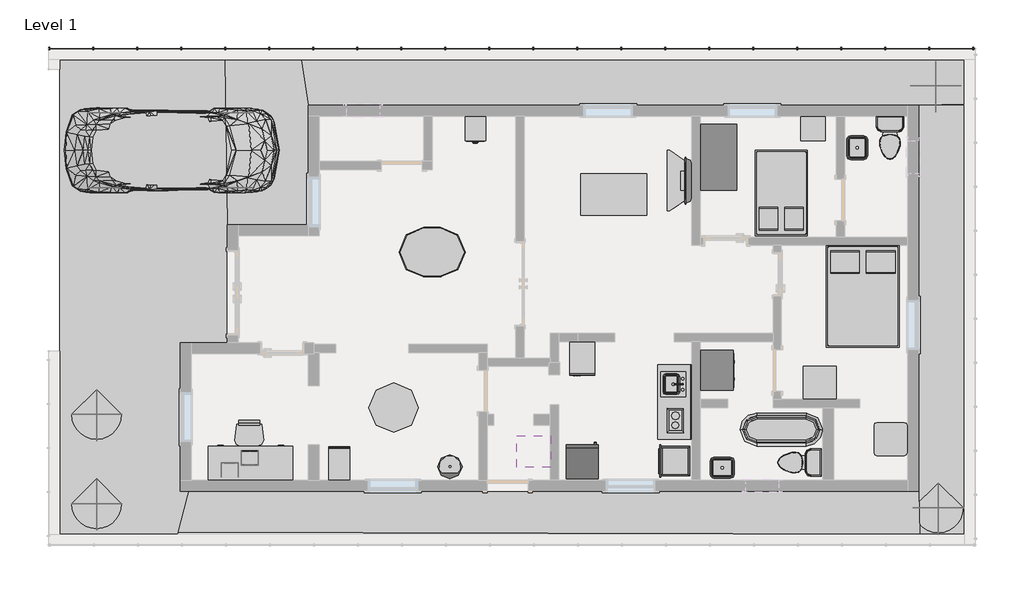
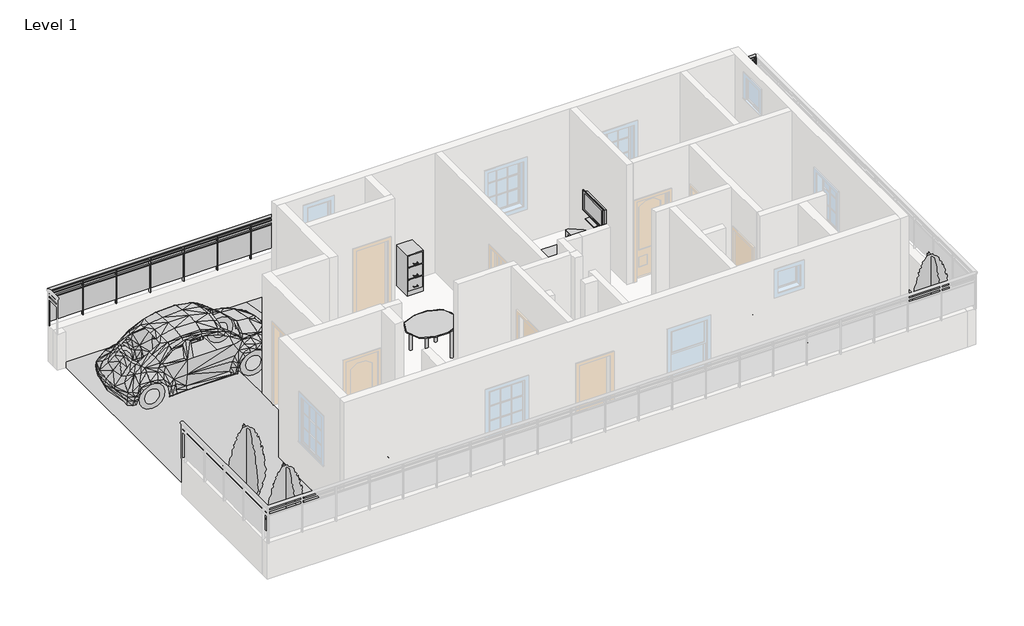
# One storey, part 3 of 3: 16 furniture elements, 15 proxies, 7 flow terminals, 4 geographic elements, 1 railing.
"""IFC4 building model written with IfcOpenShell, lengths in millimetres."""

from ifc_helpers import new_model, si_unit, point, frame, origin, place, context, project, spatial, polyline, ellipse_curve, trimmed, outline, extrude, triangles, transform, mapped, element, save
from ifc_brep_helpers import plane_surface, extruded_surface, advanced_brep
from components import entourage_4c8cfd20, proxy_db4bb64d, proxy_7e1014cc, proxy_fe84b772, proxy_a6faaae8, proxy_844211aa, proxy_8b8c2dc4, rpc_beetle_rpc_beetle_3ce7ba48, proxy_c523a7b7, flow_terminal_871c2e40, flow_terminal_d49f872f, flow_terminal_62a433f7, toilet_domestic_3d_toilet_domestic_3d_f7549cf7, toilet_domestic_3d_toilet_domestic_3d_183bbd19, flow_terminal_2ffd2f66, furniture_c8abb964, furniture_631c00ae, furniture_552c1472, chair_desk_chair_desk_ccc35c8f, furniture_b3f308bd, furniture_072f6425, furniture_08c10487, furniture_80f2079a, furniture_56245f3a, tv_stand_tv_stand_6ce107e5, furniture_e3bc833e, furniture_be1c6672, furniture_905aceb5, furniture_bcf351fa, furniture_097b63cf, furniture_5bc9ed15, rpc_tree_conifer_0001_chinese_juniper_7_1b9786cd

model = new_model("IFC4")

# Units and contexts
model_context = context("Model", 3, world=origin())
ifc_project = project(units=[si_unit("LENGTHUNIT", "METRE", prefix="MILLI")], contexts=[model_context])

# Site, building, storey
site = spatial("IfcSite", under=ifc_project)
building = spatial("IfcBuilding", under=site)
storey = spatial("IfcBuildingStorey", under=building, Name="Level 1", Elevation=0.0)

# Proxies
placement = place(None, origin())
element("IfcBuildingElementProxy", 1, Name="Building Element Proxy", at=placement, inside=storey, context=model_context, shape_type="Tessellation", body=[
    triangles([(-21898.1191772, 12173.6662354, 0.0), (-21898.1191772, 3410.6659447, 0.0), (-19722.5659241, 3410.6659447, 0.0), (-19666.685614, 6966.0811935, 0.0), (-19748.6015442, 10092.3002563, 0.0), (-18803.0848389, 6966.0811935, 0.0), (-18803.0848389, 9125.0813873, 0.0), (-18943.9727509, 10074.8350433, 0.0), (-18848.4588135, 12173.6662354, 0.0)], [[4, 1, 2], [1, 5, 9], [4, 5, 1], [2, 3, 4], [4, 6, 7], [6, 4, 3], [8, 7, 9], [8, 5, 7], [9, 5, 8], [5, 4, 7]], closed=False),
])
element("IfcBuildingElementProxy", 2, Name="Building Element Proxy", at=placement, inside=storey, context=model_context, shape_type="Tessellation", body=[
    triangles([(-18803.0848389, 9125.0813873, 0.0), (-17304.4844513, 9125.0813873, 0.0), (-17304.4844513, 11334.8813873, 0.0), (-17434.4451233, 12173.6662354, 0.0), (-18907.1703461, 12173.6662354, 0.0)], [[5, 1, 3], [5, 3, 4], [3, 1, 2]], closed=False),
])
element("IfcBuildingElementProxy", 3, Name="Building Element Proxy", at=placement, inside=storey, context=model_context, shape_type="Tessellation", body=[
    triangles([(-17304.4844513, 11334.8813873, 0.0), (-17438.9181061, 12173.6662354, 0.0), (-5184.9201462, 12173.6662354, 0.0), (-6026.8844513, 11334.8813873, 0.0), (-5184.9201462, 11344.9063568, 0.0)], [[2, 1, 4], [4, 5, 3], [4, 3, 2]], closed=False),
])
element("IfcBuildingElementProxy", 4, Name="Building Element Proxy", at=placement, inside=storey, context=model_context, shape_type="Tessellation", body=[
    triangles([(-5184.9201462, 11341.3716888, 0.0), (-6026.8844513, 11334.8813873, 0.0), (-6023.0718933, 3410.6659447, 0.0), (-5184.9201462, 3410.6659447, 0.0)], [[2, 3, 4], [4, 1, 2]], closed=False),
])
element("IfcBuildingElementProxy", 5, Name="Building Element Proxy", at=placement, inside=storey, context=model_context, shape_type="Tessellation", body=[
    triangles([(-19541.1653687, 4197.4812904, 0.0), (-19710.431781, 3439.8970093, 0.0), (-6026.8844513, 4197.4812904, 0.0), (-6033.6526428, 3410.6659447, 0.0), (-6026.8396866, 3410.6659447, 0.0), (-6011.1662247, 3410.6659447, 0.0), (-6028.8971191, 3410.6659447, 0.0)], [[2, 4, 1], [1, 4, 3], [5, 6, 3], [7, 3, 4], [3, 7, 5]], closed=False),
])
entourage_shape = entourage_4c8cfd20(model_context)
element("IfcBuildingElementProxy", 6, Name="Entourage", at=placement, inside=storey, context=model_context, shape_type="MappedRepresentation", body=[
    mapped(entourage_shape, transform((-18757.4020483, 4629.2812219, 0.0), x_axis=(1.0, 0.0, 0.0), y_axis=(0.0, 1.0, 0.0), z_axis=(0.0, 0.0, 1.0))),
])
element("IfcBuildingElementProxy", 7, Name="Entourage", at=placement, inside=storey, context=model_context, shape_type="MappedRepresentation", body=[
    mapped(entourage_shape, transform((-18387.2011117, 4781.6812219, 762.0), x_axis=(-1.0000000000000004, 0.0, 0.0), y_axis=(0.0, -1.0000000000000004, 0.0), z_axis=(0.0, 0.0, 1.0))),
])
proxy_shape = proxy_db4bb64d(model_context)
element("IfcBuildingElementProxy", 8, Name="15\" x 24\" x 34 1/2\"", ObjectType="15\" x 24\" x 34 1/2\"", at=placement, inside=storey, context=model_context, shape_type="MappedRepresentation", body=[
    mapped(proxy_shape, transform((-16464.9670881, 4969.5328437, 0.0), x_axis=(-1.0, 0.0, 0.0), y_axis=(0.0, -1.0, 0.0), z_axis=(0.0, 0.0, 1.0))),
])
proxy_2_shape = proxy_7e1014cc(model_context)
element("IfcBuildingElementProxy", 9, Name="18\" x 24\" x 34 1/2\"", ObjectType="18\" x 24\" x 34 1/2\"", at=placement, inside=storey, context=model_context, shape_type="MappedRepresentation", body=[
    mapped(proxy_2_shape, transform((-12549.6520251, 6394.8316571, 0.0), x_axis=(1.0, 0.0, 0.0), y_axis=(0.0, 1.0, 0.0), z_axis=(0.0, 0.0, 1.0))),
])
proxy_3_shape = proxy_fe84b772(model_context)
element("IfcBuildingElementProxy", 10, Name="Cook Top-2 Unit : 12\" x 18\"", ObjectType="Cook Top-2 Unit : 12\" x 18\"", at=placement, inside=storey, context=model_context, shape_type="MappedRepresentation", body=[
    mapped(proxy_3_shape, transform((-10598.8845566, 5475.3564263, 0.0), x_axis=(1.0, 0.0, 0.0), y_axis=(0.0, 1.0, 0.0), z_axis=(0.0, 0.0, 1.0))),
])
proxy_4_shape = proxy_a6faaae8(model_context)
element("IfcBuildingElementProxy", 11, Name="Cook Top-4 Unit2 : 22\" x 20\"", ObjectType="Cook Top-4 Unit2 : 22\" x 20\"", at=placement, inside=storey, context=model_context, shape_type="MappedRepresentation", body=[
    mapped(proxy_4_shape, transform((-13138.8845566, 4934.0812219, 914.4), x_axis=(1.0, 0.0, 0.0), y_axis=(0.0, 1.0, 0.0), z_axis=(0.0, 0.0, 1.0))),
])
proxy_5_shape = proxy_844211aa(model_context)
element("IfcBuildingElementProxy", 12, Name="Kitchenette - Small : 54\"", ObjectType="Kitchenette - Small : 54\"", at=placement, inside=storey, context=model_context, shape_type="MappedRepresentation", body=[
    mapped(proxy_5_shape, transform((-10217.8845566, 5867.2189268, 0.0), x_axis=(0.0, -1.0, 0.0), y_axis=(1.0, 0.0, 0.0), z_axis=(0.0, 0.0, 1.0))),
])
proxy_6_shape = proxy_8b8c2dc4(model_context)
element("IfcBuildingElementProxy", 13, Name="Oven Double-Built-in : 21 1/2\" x 39 1/4\" x 21\"", ObjectType="Oven Double-Built-in : 21 1/2\" x 39 1/4\" x 21\"", at=placement, inside=storey, context=model_context, shape_type="MappedRepresentation", body=[
    mapped(proxy_6_shape, transform((-10663.7504156, 4721.1062946, 0.0), x_axis=(0.0, -1.0000000000000004, 0.0), y_axis=(1.0000000000000004, 0.0, 0.0), z_axis=(0.0, 0.0, 1.0))),
])
rpc_beetle_rpc_beetle_shape = rpc_beetle_rpc_beetle_3ce7ba48(model_context)
element("IfcBuildingElementProxy", 14, Name="RPC Beetle : RPC Beetle", ObjectType="RPC Beetle : RPC Beetle", at=placement, inside=storey, context=model_context, shape_type="MappedRepresentation", body=[
    mapped(rpc_beetle_rpc_beetle_shape, transform((-21063.6845566, 10496.6812219, 0.0), x_axis=(0.0, -1.0000000000000002, 0.0), y_axis=(1.0000000000000002, 0.0, 0.0), z_axis=(0.0, 0.0, 1.0))),
])
proxy_7_shape = proxy_c523a7b7(model_context)
element("IfcBuildingElementProxy", 15, Name="Refrigerator : 24\" x 25\" LH", ObjectType="Refrigerator : 24\" x 25\" LH", at=placement, inside=storey, context=model_context, shape_type="MappedRepresentation", body=[
    mapped(proxy_7_shape, transform((-12243.5345566, 4729.6822504, 0.0), x_axis=(-1.0000000000000004, 0.0, 0.0), y_axis=(0.0, -1.0000000000000004, 0.0), z_axis=(0.0, 0.0, 1.0))),
])

# Flow terminals
flow_terminal_shape = flow_terminal_871c2e40(model_context)
element("IfcFlowTerminal", 16, ObjectType="Sink Kitchen-Island : 18\" x 18\"", at=placement, inside=storey, context=model_context, shape_type="MappedRepresentation", body=[
    mapped(flow_terminal_shape, transform((-10563.1299577, 6194.3704625, 0.0), x_axis=(0.0, -1.0, 0.0), y_axis=(1.0, 0.0, 0.0), z_axis=(0.0, 0.0, 1.0))),
])
flow_terminal_2_shape = flow_terminal_d49f872f(model_context)
element("IfcFlowTerminal", 17, ObjectType="Sink Vanity-Round : 19\" x 19\"", at=placement, inside=storey, context=model_context, shape_type="MappedRepresentation", body=[
    mapped(flow_terminal_2_shape, transform((-14591.632816, 4740.1488915, 482.6), x_axis=(-1.0000000000000004, 0.0, 0.0), y_axis=(0.0, -1.0000000000000004, 0.0), z_axis=(0.0, 0.0, 1.0))),
])
flow_terminal_3_shape = flow_terminal_62a433f7(model_context)
element("IfcFlowTerminal", 18, ObjectType="Sink Vanity-Square : 20\" x 18\"", at=placement, inside=storey, context=model_context, shape_type="MappedRepresentation", body=[
    mapped(flow_terminal_3_shape, transform((-9643.395316, 4580.826623, 609.6), x_axis=(-1.0000000000000002, 0.0, 0.0), y_axis=(0.0, -1.0000000000000002, 0.0), z_axis=(0.0, 0.0, 1.0))),
])
element("IfcFlowTerminal", 19, ObjectType="Sink Vanity-Square : 20\" x 18\"", at=placement, inside=storey, context=model_context, shape_type="MappedRepresentation", body=[
    mapped(flow_terminal_3_shape, transform((-7218.3391555, 10531.7919813, 609.6), x_axis=(0.0, 1.0000000000000004, 0.0), y_axis=(-1.0000000000000004, 0.0, 0.0), z_axis=(0.0, 0.0, 1.0))),
])
toilet_domestic_3d_toilet_domestic_3d_shape = toilet_domestic_3d_toilet_domestic_3d_f7549cf7(model_context)
toilet_domestic_3d_toilet_domestic_3d_2_shape = toilet_domestic_3d_toilet_domestic_3d_183bbd19(model_context)
element("IfcFlowTerminal", 20, ObjectType="Toilet-Domestic-3D : Toilet-Domestic-3D", at=placement, inside=storey, context=model_context, shape_type="MappedRepresentation", body=[
    mapped(toilet_domestic_3d_toilet_domestic_3d_shape, transform((-8324.980584, 4730.8812219, 0.0), x_axis=(0.0, -1.0000000000000004, 0.0), y_axis=(1.0000000000000004, 0.0, 0.0), z_axis=(0.0, 0.0, 1.0))),
    mapped(toilet_domestic_3d_toilet_domestic_3d_2_shape, transform((-8324.980584, 4730.8812219, 0.0), x_axis=(0.0, -1.0000000000000004, 0.0), y_axis=(1.0000000000000004, 0.0, 0.0), z_axis=(0.0, 0.0, 1.0))),
])
element("IfcFlowTerminal", 21, ObjectType="Toilet-Domestic-3D : Toilet-Domestic-3D", at=placement, inside=storey, context=model_context, shape_type="MappedRepresentation", body=[
    mapped(toilet_domestic_3d_toilet_domestic_3d_shape, transform((-6560.2845566, 10636.9851945, 0.0), x_axis=(1.0, 0.0, 0.0), y_axis=(0.0, 1.0, 0.0), z_axis=(0.0, 0.0, 1.0))),
    mapped(toilet_domestic_3d_toilet_domestic_3d_2_shape, transform((-6560.2845566, 10636.9851945, 0.0), x_axis=(1.0, 0.0, 0.0), y_axis=(0.0, 1.0, 0.0), z_axis=(0.0, 0.0, 1.0))),
])
flow_terminal_4_shape = flow_terminal_2ffd2f66(model_context)
element("IfcFlowTerminal", 22, ObjectType="Tub-Free Standing-3D : 30\" x 60\"", at=placement, inside=storey, context=model_context, shape_type="MappedRepresentation", body=[
    mapped(flow_terminal_4_shape, transform((-8566.8845566, 5340.4812219, 0.0), x_axis=(0.0, -0.9999999999999998, 0.0), y_axis=(0.9999999999999998, 0.0, 0.0), z_axis=(0.0, 0.0, 1.0))),
])

# Furniture
furniture_shape = furniture_c8abb964(model_context)
element("IfcFurniture", 23, ObjectType="Bed-Box : Double 53\" x 74\"", at=placement, inside=storey, context=model_context, shape_type="MappedRepresentation", body=[
    mapped(furniture_shape, transform((-7398.4845566, 8038.7107301, 0.0), x_axis=(1.0, 0.0, 0.0), y_axis=(0.0, 1.0, 0.0), z_axis=(0.0, 0.0, 1.0))),
])
furniture_2_shape = furniture_631c00ae(model_context)
element("IfcFurniture", 24, ObjectType="Bed-Box : Twin 38\" x 74\"", at=placement, inside=storey, context=model_context, shape_type="MappedRepresentation", body=[
    mapped(furniture_2_shape, transform((-8227.7320976, 9474.8517137, 0.0), x_axis=(-1.0, 0.0, 0.0), y_axis=(0.0, -1.0, 0.0), z_axis=(0.0, 0.0, 1.0))),
])
furniture_3_shape = furniture_552c1472(model_context)
element("IfcFurniture", 25, ObjectType="Cabinet-File 3 Drawer : 15\" x 18\"", at=placement, inside=storey, context=model_context, shape_type="MappedRepresentation", body=[
    mapped(furniture_3_shape, transform((-14090.4881096, 11045.215522, 0.0), x_axis=(1.0, 0.0, 0.0), y_axis=(0.0, 1.0, 0.0), z_axis=(0.0, 0.0, 1.0))),
])
chair_desk_chair_desk_shape = chair_desk_chair_desk_ccc35c8f(model_context)
element("IfcFurniture", 26, ObjectType="Chair-Desk : Chair-Desk", at=placement, inside=storey, context=model_context, shape_type="MappedRepresentation", body=[
    mapped(chair_desk_chair_desk_shape, transform((-18396.6845566, 5442.0812219, 0.0), x_axis=(-1.0, 0.0, 0.0), y_axis=(0.0, -1.0, 0.0), z_axis=(0.0, 0.0, 1.0))),
])
furniture_4_shape = furniture_b3f308bd(model_context)
element("IfcFurniture", 27, ObjectType="Counter Top w Sink Hole : 24\" Depth", at=placement, inside=storey, context=model_context, shape_type="MappedRepresentation", body=[
    mapped(furniture_4_shape, transform((-10217.8845566, 5333.8189268, 0.0), x_axis=(0.0, -1.0, 0.0), y_axis=(1.0, 0.0, 0.0), z_axis=(0.0, 0.0, 1.0))),
])
furniture_5_shape = furniture_072f6425(model_context)
element("IfcFurniture", 28, ObjectType="Desk : 60\" x 30\"", at=placement, inside=storey, context=model_context, shape_type="MappedRepresentation", body=[
    mapped(furniture_5_shape, transform((-19133.2845566, 4248.2812219, 0.0), x_axis=(1.0000000000000007, 0.0, 0.0), y_axis=(0.0, 1.0000000000000007, 0.0), z_axis=(0.0, 0.0, 1.0))),
])
furniture_6_shape = furniture_08c10487(model_context)
element("IfcFurniture", 29, ObjectType="Dresser.0001 : 48\" x 60\" x 24\"", at=placement, inside=storey, context=model_context, shape_type="MappedRepresentation", body=[
    mapped(furniture_6_shape, transform((-10123.8475107, 6701.8744817, 0.0), x_axis=(0.0, 1.0000000000000002, 0.0), y_axis=(-1.0000000000000002, 0.0, 0.0), z_axis=(0.0, 0.0, 1.0))),
])
furniture_7_shape = furniture_80f2079a(model_context)
element("IfcFurniture", 30, ObjectType="Entertainment Center : 72\" x 72\" x 24\"", at=placement, inside=storey, context=model_context, shape_type="MappedRepresentation", body=[
    mapped(furniture_7_shape, transform((-10167.0845566, 10369.6812219, 0.0), x_axis=(0.0, 1.0000000000000002, 0.0), y_axis=(-1.0000000000000002, 0.0, 0.0), z_axis=(0.0, 0.0, 1.0))),
])
furniture_8_shape = furniture_56245f3a(model_context)
element("IfcFurniture", 31, ObjectType="TV - Flat Screen : 32\"", at=placement, inside=storey, context=model_context, shape_type="MappedRepresentation", body=[
    mapped(furniture_8_shape, transform((-10276.4231803, 9933.9367078, 914.4), x_axis=(0.0, -1.0000000000000002, 0.0), y_axis=(1.0000000000000002, 0.0, 0.0), z_axis=(0.0, 0.0, 1.0))),
])
tv_stand_tv_stand_shape = tv_stand_tv_stand_6ce107e5(model_context)
element("IfcFurniture", 32, ObjectType="TV Stand : TV Stand", at=placement, inside=storey, context=model_context, shape_type="MappedRepresentation", body=[
    mapped(tv_stand_tv_stand_shape, transform((-10217.8845566, 10063.069224, 0.0), x_axis=(0.0, -1.0000000000000004, 0.0), y_axis=(1.0000000000000004, 0.0, 0.0), z_axis=(0.0, 0.0, 1.0))),
])
furniture_9_shape = furniture_e3bc833e(model_context)
element("IfcFurniture", 33, ObjectType="Table-Dining : 30\" x 84\" x 22\"", at=placement, inside=storey, context=model_context, shape_type="MappedRepresentation", body=[
    mapped(furniture_9_shape, transform((-11683.9503233, 9588.6701441, 0.0), x_axis=(1.0, 0.0, 0.0), y_axis=(0.0, 1.0, 0.0), z_axis=(0.0, 0.0, 1.0))),
])
furniture_10_shape = furniture_be1c6672(model_context)
element("IfcFurniture", 34, ObjectType="Table-Dining Oval : 36\" x 48\"", at=placement, inside=storey, context=model_context, shape_type="MappedRepresentation", body=[
    mapped(furniture_10_shape, transform((-14616.6648845, 8975.1795826, 0.0), x_axis=(1.0, 0.0, 0.0), y_axis=(0.0, 1.0, 0.0), z_axis=(0.0, 0.0, 1.0))),
])
furniture_11_shape = furniture_905aceb5(model_context)
element("IfcFurniture", 35, ObjectType="Table-Dining Round w Chairs : 36\" Diameter", at=placement, inside=storey, context=model_context, shape_type="MappedRepresentation", body=[
    mapped(furniture_11_shape, transform((-15833.3665238, 5931.7599104, 0.0), x_axis=(1.0, 0.0, 0.0), y_axis=(0.0, 1.0, 0.0), z_axis=(0.0, 0.0, 1.0))),
])
furniture_12_shape = furniture_bcf351fa(model_context)
element("IfcFurniture", 36, ObjectType="Table-End : 24\" x 24\"", at=placement, inside=storey, context=model_context, shape_type="MappedRepresentation", body=[
    mapped(furniture_12_shape, transform((-6856.1181869, 5010.2812219, 0.0), x_axis=(1.0, 0.0, 0.0), y_axis=(0.0, 1.0, 0.0), z_axis=(0.0, 0.0, 1.0))),
])
furniture_13_shape = furniture_097b63cf(model_context)
element("IfcFurniture", 37, ObjectType="Table-Night Stand : 18\" x 18\" x 24\"", at=placement, inside=storey, context=model_context, shape_type="MappedRepresentation", body=[
    mapped(furniture_13_shape, transform((-8215.0181869, 10674.4812219, 0.0), x_axis=(1.0, 0.0, 0.0), y_axis=(0.0, 1.0, 0.0), z_axis=(0.0, 0.0, 1.0))),
])
furniture_14_shape = furniture_5bc9ed15(model_context)
element("IfcFurniture", 38, ObjectType="Table-Night Stand : 24\" x 24\" x 30\"", at=placement, inside=storey, context=model_context, shape_type="MappedRepresentation", body=[
    mapped(furniture_14_shape, transform((-8164.2181869, 5899.2812219, 0.0), x_axis=(1.0, 0.0, 0.0), y_axis=(0.0, 1.0, 0.0), z_axis=(0.0, 0.0, 1.0))),
])

# Geographic elements
rpc_tree_conifer_0001_chinese_juniper_7_shape = rpc_tree_conifer_0001_chinese_juniper_7_1b9786cd(model_context)
element("IfcGeographicElement", 39, ObjectType="RPC Tree - Conifer.0001 : Chinese Juniper - 7'", at=placement, inside=storey, context=model_context, shape_type="MappedRepresentation", body=[
    mapped(rpc_tree_conifer_0001_chinese_juniper_7_shape, transform((-21216.2812277, 3968.8812219, 0.0), x_axis=(1.0, 0.0, 0.0), y_axis=(0.0, 1.0, 0.0), z_axis=(0.0, 0.0, 1.0))),
])
element("IfcGeographicElement", 40, ObjectType="RPC Tree - Conifer.0001 : Chinese Juniper - 7'", at=placement, inside=storey, context=model_context, shape_type="MappedRepresentation", body=[
    mapped(rpc_tree_conifer_0001_chinese_juniper_7_shape, transform((-21216.2812277, 5619.8812219, 0.0), x_axis=(1.0, 0.0, 0.0), y_axis=(0.0, 1.0, 0.0), z_axis=(0.0, 0.0, 1.0))),
])
element("IfcGeographicElement", 41, ObjectType="RPC Tree - Conifer.0001 : Chinese Juniper - 7'", at=placement, inside=storey, context=model_context, shape_type="MappedRepresentation", body=[
    mapped(rpc_tree_conifer_0001_chinese_juniper_7_shape, transform((-5667.7169317, 3892.6812219, 0.0), x_axis=(1.0, 0.0, 0.0), y_axis=(0.0, 1.0, 0.0), z_axis=(0.0, 0.0, 1.0))),
])
element("IfcGeographicElement", 42, ObjectType="RPC Tree - Conifer.0001 : Chinese Juniper - 7'", at=placement, inside=storey, context=model_context, shape_type="MappedRepresentation", body=[
    mapped(rpc_tree_conifer_0001_chinese_juniper_7_shape, transform((-5718.5169317, 11691.0658827, 0.0), x_axis=(1.0, 0.0, 0.0), y_axis=(0.0, 1.0, 0.0), z_axis=(0.0, 0.0, 1.0))),
])

# Railing
element("IfcRailing", 43, ObjectType="Glass Panel - Bottom Fill", at=placement, inside=storey, context=model_context, shape_type="SolidModel", body=[
    advanced_brep(
    [(-5007.1202606, 12338.7658827, 1828.8), (-5007.1202606, 12414.9658827, 1828.8), (-22101.3202606, 12338.7658827, 1828.8), (-22101.3202606, 12414.9658827, 1828.8)],
    [
        (0, 1, ellipse_curve(frame((-5007.1202606, 12376.8658827, 1828.8), z_axis=(1.0, 0.0, 0.0), x_axis=(0.0, 1.0, 0.0)), 38.1, 28.575)),
        (1, 0, ellipse_curve(frame((-5007.1202606, 12376.8658827, 1828.8), z_axis=(1.0, 0.0, 0.0), x_axis=(0.0, 1.0, 0.0)), 38.1, 28.575)),
        (2, 3, ellipse_curve(frame((-22101.3202606, 12376.8658827, 1828.8), z_axis=(-1.0, 0.0, 0.0), x_axis=(0.0, 1.0, 0.0)), 38.1, 28.575)),
        (3, 2, ellipse_curve(frame((-22101.3202606, 12376.8658827, 1828.8), z_axis=(-1.0, 0.0, 0.0), x_axis=(0.0, 1.0, 0.0)), 38.1, 28.575)),
        (0, 2),
        (3, 1),
    ],
    [
        plane_surface(frame((-5007.1202606, 12376.8658827, 1828.8), z_axis=(1.0, 0.0, 0.0), x_axis=(0.0, -1.0, 0.0))),
        plane_surface(frame((-22101.3202606, 12376.8658827, 1828.8), z_axis=(-1.0, 0.0, 0.0), x_axis=(0.0, -1.0, 0.0))),
        extruded_surface(trimmed(ellipse_curve(frame((-22101.3202606, 12376.8658827, 1828.8), z_axis=(1.0, 0.0, 0.0), x_axis=(0.0, 1.0, 0.0)), 38.1, 28.575), [point((-22101.3202606, 12338.7658827, 1828.8))], [point((-22101.3202606, 12414.9658827, 1828.8))], True, "CARTESIAN"), (17094.2, 0.0, 0.0), 17094.2),
        extruded_surface(trimmed(ellipse_curve(frame((-22101.3202606, 12376.8658827, 1828.8), z_axis=(1.0, 0.0, 0.0), x_axis=(0.0, 1.0, 0.0)), 38.1, 28.575), [point((-22101.3202606, 12414.9658827, 1828.8))], [point((-22101.3202606, 12338.7658827, 1828.8))], True, "CARTESIAN"), (17094.2, 0.0, 0.0), 17094.2),
    ],
    [
        (0, [[1, 2]]),
        (1, [[3, 4]]),
        (2, [[-1, 5, -4, 6]]),
        (3, [[-2, -6, -3, -5]]),
    ],
),
    extrude(outline(polyline([(-5007.1202606, 12389.5658827), (-5007.1202606, 12364.1658827), (-22101.3202606, 12364.1658827), (-22101.3202606, 12389.5658827), (-5007.1202606, 12389.5658827)])), frame((0.0, 0.0, 1714.5), z_axis=(0.0, 0.0, 1.0), x_axis=(1.0, 0.0, 0.0)), (0.0, 0.0, 1.0), 25.4),
    extrude(outline(polyline([(-5007.1202606, 12389.5658827), (-5007.1202606, 12364.1658827), (-22101.3202606, 12364.1658827), (-22101.3202606, 12389.5658827), (-5007.1202606, 12389.5658827)])), frame((0.0, 0.0, 1612.9), z_axis=(0.0, 0.0, 1.0), x_axis=(1.0, 0.0, 0.0)), (0.0, 0.0, 1.0), 25.4),
    extrude(outline(polyline([(-22082.2702606, 12402.2658827), (-22082.2702606, 12351.4658827), (-22094.9702606, 12351.4658827), (-22094.9702606, 12402.2658827), (-22082.2702606, 12402.2658827)])), frame((0.0, 0.0, 914.4), z_axis=(0.0, 0.0, 1.0), x_axis=(1.0, 0.0, 0.0)), (0.0, 0.0, 1.0), 885.6788223),
    extrude(outline(polyline([(-21275.8202606, 12370.3307257), (-22088.6202606, 12370.3307257), (-22088.6202606, 12376.6807257), (-21275.8202606, 12376.6807257), (-21275.8202606, 12370.3307257)])), frame((0.0, 0.0, 1016.0), z_axis=(0.0, 0.0, 1.0), x_axis=(1.0, 0.0, 0.0)), (0.0, 0.0, 1.0), 596.9),
    extrude(outline(polyline([(-21269.4702606, 12402.2658827), (-21269.4702606, 12351.4658827), (-21282.1702606, 12351.4658827), (-21282.1702606, 12402.2658827), (-21269.4702606, 12402.2658827)])), frame((0.0, 0.0, 914.4), z_axis=(0.0, 0.0, 1.0), x_axis=(1.0, 0.0, 0.0)), (0.0, 0.0, 1.0), 885.6788223),
    extrude(outline(polyline([(-20463.0202606, 12370.3307257), (-21275.8202606, 12370.3307257), (-21275.8202606, 12376.6807257), (-20463.0202606, 12376.6807257), (-20463.0202606, 12370.3307257)])), frame((0.0, 0.0, 1016.0), z_axis=(0.0, 0.0, 1.0), x_axis=(1.0, 0.0, 0.0)), (0.0, 0.0, 1.0), 596.9),
    extrude(outline(polyline([(-20456.6702606, 12402.2658827), (-20456.6702606, 12351.4658827), (-20469.3702606, 12351.4658827), (-20469.3702606, 12402.2658827), (-20456.6702606, 12402.2658827)])), frame((0.0, 0.0, 914.4), z_axis=(0.0, 0.0, 1.0), x_axis=(1.0, 0.0, 0.0)), (0.0, 0.0, 1.0), 885.6788223),
    extrude(outline(polyline([(-19650.2202606, 12370.3307257), (-20463.0202606, 12370.3307257), (-20463.0202606, 12376.6807257), (-19650.2202606, 12376.6807257), (-19650.2202606, 12370.3307257)])), frame((0.0, 0.0, 1016.0), z_axis=(0.0, 0.0, 1.0), x_axis=(1.0, 0.0, 0.0)), (0.0, 0.0, 1.0), 596.9),
    extrude(outline(polyline([(-19643.8702606, 12402.2658827), (-19643.8702606, 12351.4658827), (-19656.5702606, 12351.4658827), (-19656.5702606, 12402.2658827), (-19643.8702606, 12402.2658827)])), frame((0.0, 0.0, 914.4), z_axis=(0.0, 0.0, 1.0), x_axis=(1.0, 0.0, 0.0)), (0.0, 0.0, 1.0), 885.6788223),
    extrude(outline(polyline([(-18837.4202606, 12370.3307257), (-19650.2202606, 12370.3307257), (-19650.2202606, 12376.6807257), (-18837.4202606, 12376.6807257), (-18837.4202606, 12370.3307257)])), frame((0.0, 0.0, 1016.0), z_axis=(0.0, 0.0, 1.0), x_axis=(1.0, 0.0, 0.0)), (0.0, 0.0, 1.0), 596.9),
    extrude(outline(polyline([(-18831.0702606, 12402.2658827), (-18831.0702606, 12351.4658827), (-18843.7702606, 12351.4658827), (-18843.7702606, 12402.2658827), (-18831.0702606, 12402.2658827)])), frame((0.0, 0.0, 914.4), z_axis=(0.0, 0.0, 1.0), x_axis=(1.0, 0.0, 0.0)), (0.0, 0.0, 1.0), 885.6788223),
    extrude(outline(polyline([(-18024.6202606, 12370.3307257), (-18837.4202606, 12370.3307257), (-18837.4202606, 12376.6807257), (-18024.6202606, 12376.6807257), (-18024.6202606, 12370.3307257)])), frame((0.0, 0.0, 1016.0), z_axis=(0.0, 0.0, 1.0), x_axis=(1.0, 0.0, 0.0)), (0.0, 0.0, 1.0), 596.9),
    extrude(outline(polyline([(-18018.2702606, 12402.2658827), (-18018.2702606, 12351.4658827), (-18030.9702606, 12351.4658827), (-18030.9702606, 12402.2658827), (-18018.2702606, 12402.2658827)])), frame((0.0, 0.0, 914.4), z_axis=(0.0, 0.0, 1.0), x_axis=(1.0, 0.0, 0.0)), (0.0, 0.0, 1.0), 885.6788223),
    extrude(outline(polyline([(-17211.8202606, 12370.3307257), (-18024.6202606, 12370.3307257), (-18024.6202606, 12376.6807257), (-17211.8202606, 12376.6807257), (-17211.8202606, 12370.3307257)])), frame((0.0, 0.0, 1016.0), z_axis=(0.0, 0.0, 1.0), x_axis=(1.0, 0.0, 0.0)), (0.0, 0.0, 1.0), 596.9),
    extrude(outline(polyline([(-17205.4702606, 12402.2658827), (-17205.4702606, 12351.4658827), (-17218.1702606, 12351.4658827), (-17218.1702606, 12402.2658827), (-17205.4702606, 12402.2658827)])), frame((0.0, 0.0, 914.4), z_axis=(0.0, 0.0, 1.0), x_axis=(1.0, 0.0, 0.0)), (0.0, 0.0, 1.0), 885.6788223),
    extrude(outline(polyline([(-16399.0202606, 12370.3307257), (-17211.8202606, 12370.3307257), (-17211.8202606, 12376.6807257), (-16399.0202606, 12376.6807257), (-16399.0202606, 12370.3307257)])), frame((0.0, 0.0, 1016.0), z_axis=(0.0, 0.0, 1.0), x_axis=(1.0, 0.0, 0.0)), (0.0, 0.0, 1.0), 596.9),
    extrude(outline(polyline([(-16392.6702606, 12402.2658827), (-16392.6702606, 12351.4658827), (-16405.3702606, 12351.4658827), (-16405.3702606, 12402.2658827), (-16392.6702606, 12402.2658827)])), frame((0.0, 0.0, 914.4), z_axis=(0.0, 0.0, 1.0), x_axis=(1.0, 0.0, 0.0)), (0.0, 0.0, 1.0), 885.6788223),
    extrude(outline(polyline([(-15586.2202606, 12370.3307257), (-16399.0202606, 12370.3307257), (-16399.0202606, 12376.6807257), (-15586.2202606, 12376.6807257), (-15586.2202606, 12370.3307257)])), frame((0.0, 0.0, 1016.0), z_axis=(0.0, 0.0, 1.0), x_axis=(1.0, 0.0, 0.0)), (0.0, 0.0, 1.0), 596.9),
    extrude(outline(polyline([(-15579.8702606, 12402.2658827), (-15579.8702606, 12351.4658827), (-15592.5702606, 12351.4658827), (-15592.5702606, 12402.2658827), (-15579.8702606, 12402.2658827)])), frame((0.0, 0.0, 914.4), z_axis=(0.0, 0.0, 1.0), x_axis=(1.0, 0.0, 0.0)), (0.0, 0.0, 1.0), 885.6788223),
    extrude(outline(polyline([(-14773.4202606, 12370.3307257), (-15586.2202606, 12370.3307257), (-15586.2202606, 12376.6807257), (-14773.4202606, 12376.6807257), (-14773.4202606, 12370.3307257)])), frame((0.0, 0.0, 1016.0), z_axis=(0.0, 0.0, 1.0), x_axis=(1.0, 0.0, 0.0)), (0.0, 0.0, 1.0), 596.9),
    extrude(outline(polyline([(-14767.0702606, 12402.2658827), (-14767.0702606, 12351.4658827), (-14779.7702606, 12351.4658827), (-14779.7702606, 12402.2658827), (-14767.0702606, 12402.2658827)])), frame((0.0, 0.0, 914.4), z_axis=(0.0, 0.0, 1.0), x_axis=(1.0, 0.0, 0.0)), (0.0, 0.0, 1.0), 885.6788223),
    extrude(outline(polyline([(-13960.6202606, 12370.3307257), (-14773.4202606, 12370.3307257), (-14773.4202606, 12376.6807257), (-13960.6202606, 12376.6807257), (-13960.6202606, 12370.3307257)])), frame((0.0, 0.0, 1016.0), z_axis=(0.0, 0.0, 1.0), x_axis=(1.0, 0.0, 0.0)), (0.0, 0.0, 1.0), 596.9),
    extrude(outline(polyline([(-13954.2702606, 12402.2658827), (-13954.2702606, 12351.4658827), (-13966.9702606, 12351.4658827), (-13966.9702606, 12402.2658827), (-13954.2702606, 12402.2658827)])), frame((0.0, 0.0, 914.4), z_axis=(0.0, 0.0, 1.0), x_axis=(1.0, 0.0, 0.0)), (0.0, 0.0, 1.0), 885.6788223),
    extrude(outline(polyline([(-13147.8202606, 12370.3307257), (-13960.6202606, 12370.3307257), (-13960.6202606, 12376.6807257), (-13147.8202606, 12376.6807257), (-13147.8202606, 12370.3307257)])), frame((0.0, 0.0, 1016.0), z_axis=(0.0, 0.0, 1.0), x_axis=(1.0, 0.0, 0.0)), (0.0, 0.0, 1.0), 596.9),
    extrude(outline(polyline([(-13141.4702606, 12402.2658827), (-13141.4702606, 12351.4658827), (-13154.1702606, 12351.4658827), (-13154.1702606, 12402.2658827), (-13141.4702606, 12402.2658827)])), frame((0.0, 0.0, 914.4), z_axis=(0.0, 0.0, 1.0), x_axis=(1.0, 0.0, 0.0)), (0.0, 0.0, 1.0), 885.6788223),
    extrude(outline(polyline([(-12335.0202606, 12370.3307257), (-13147.8202606, 12370.3307257), (-13147.8202606, 12376.6807257), (-12335.0202606, 12376.6807257), (-12335.0202606, 12370.3307257)])), frame((0.0, 0.0, 1016.0), z_axis=(0.0, 0.0, 1.0), x_axis=(1.0, 0.0, 0.0)), (0.0, 0.0, 1.0), 596.9),
    extrude(outline(polyline([(-12328.6702606, 12402.2658827), (-12328.6702606, 12351.4658827), (-12341.3702606, 12351.4658827), (-12341.3702606, 12402.2658827), (-12328.6702606, 12402.2658827)])), frame((0.0, 0.0, 914.4), z_axis=(0.0, 0.0, 1.0), x_axis=(1.0, 0.0, 0.0)), (0.0, 0.0, 1.0), 885.6788223),
    extrude(outline(polyline([(-11522.2202606, 12370.3307257), (-12335.0202606, 12370.3307257), (-12335.0202606, 12376.6807257), (-11522.2202606, 12376.6807257), (-11522.2202606, 12370.3307257)])), frame((0.0, 0.0, 1016.0), z_axis=(0.0, 0.0, 1.0), x_axis=(1.0, 0.0, 0.0)), (0.0, 0.0, 1.0), 596.9),
    extrude(outline(polyline([(-11515.8702606, 12402.2658827), (-11515.8702606, 12351.4658827), (-11528.5702606, 12351.4658827), (-11528.5702606, 12402.2658827), (-11515.8702606, 12402.2658827)])), frame((0.0, 0.0, 914.4), z_axis=(0.0, 0.0, 1.0), x_axis=(1.0, 0.0, 0.0)), (0.0, 0.0, 1.0), 885.6788223),
    extrude(outline(polyline([(-10709.4202606, 12370.3307257), (-11522.2202606, 12370.3307257), (-11522.2202606, 12376.6807257), (-10709.4202606, 12376.6807257), (-10709.4202606, 12370.3307257)])), frame((0.0, 0.0, 1016.0), z_axis=(0.0, 0.0, 1.0), x_axis=(1.0, 0.0, 0.0)), (0.0, 0.0, 1.0), 596.9),
    extrude(outline(polyline([(-10703.0702606, 12402.2658827), (-10703.0702606, 12351.4658827), (-10715.7702606, 12351.4658827), (-10715.7702606, 12402.2658827), (-10703.0702606, 12402.2658827)])), frame((0.0, 0.0, 914.4), z_axis=(0.0, 0.0, 1.0), x_axis=(1.0, 0.0, 0.0)), (0.0, 0.0, 1.0), 885.6788223),
    extrude(outline(polyline([(-9896.6202606, 12370.3307257), (-10709.4202606, 12370.3307257), (-10709.4202606, 12376.6807257), (-9896.6202606, 12376.6807257), (-9896.6202606, 12370.3307257)])), frame((0.0, 0.0, 1016.0), z_axis=(0.0, 0.0, 1.0), x_axis=(1.0, 0.0, 0.0)), (0.0, 0.0, 1.0), 596.9),
    extrude(outline(polyline([(-9890.2702606, 12402.2658827), (-9890.2702606, 12351.4658827), (-9902.9702606, 12351.4658827), (-9902.9702606, 12402.2658827), (-9890.2702606, 12402.2658827)])), frame((0.0, 0.0, 914.4), z_axis=(0.0, 0.0, 1.0), x_axis=(1.0, 0.0, 0.0)), (0.0, 0.0, 1.0), 885.6788223),
    extrude(outline(polyline([(-9083.8202606, 12370.3307257), (-9896.6202606, 12370.3307257), (-9896.6202606, 12376.6807257), (-9083.8202606, 12376.6807257), (-9083.8202606, 12370.3307257)])), frame((0.0, 0.0, 1016.0), z_axis=(0.0, 0.0, 1.0), x_axis=(1.0, 0.0, 0.0)), (0.0, 0.0, 1.0), 596.9),
    extrude(outline(polyline([(-9077.4702606, 12402.2658827), (-9077.4702606, 12351.4658827), (-9090.1702606, 12351.4658827), (-9090.1702606, 12402.2658827), (-9077.4702606, 12402.2658827)])), frame((0.0, 0.0, 914.4), z_axis=(0.0, 0.0, 1.0), x_axis=(1.0, 0.0, 0.0)), (0.0, 0.0, 1.0), 885.6788223),
    extrude(outline(polyline([(-8271.0202606, 12370.3307257), (-9083.8202606, 12370.3307257), (-9083.8202606, 12376.6807257), (-8271.0202606, 12376.6807257), (-8271.0202606, 12370.3307257)])), frame((0.0, 0.0, 1016.0), z_axis=(0.0, 0.0, 1.0), x_axis=(1.0, 0.0, 0.0)), (0.0, 0.0, 1.0), 596.9),
    extrude(outline(polyline([(-8264.6702606, 12402.2658827), (-8264.6702606, 12351.4658827), (-8277.3702606, 12351.4658827), (-8277.3702606, 12402.2658827), (-8264.6702606, 12402.2658827)])), frame((0.0, 0.0, 914.4), z_axis=(0.0, 0.0, 1.0), x_axis=(1.0, 0.0, 0.0)), (0.0, 0.0, 1.0), 885.6788223),
    extrude(outline(polyline([(-7458.2202606, 12370.3307257), (-8271.0202606, 12370.3307257), (-8271.0202606, 12376.6807257), (-7458.2202606, 12376.6807257), (-7458.2202606, 12370.3307257)])), frame((0.0, 0.0, 1016.0), z_axis=(0.0, 0.0, 1.0), x_axis=(1.0, 0.0, 0.0)), (0.0, 0.0, 1.0), 596.9),
    extrude(outline(polyline([(-7451.8702606, 12402.2658827), (-7451.8702606, 12351.4658827), (-7464.5702606, 12351.4658827), (-7464.5702606, 12402.2658827), (-7451.8702606, 12402.2658827)])), frame((0.0, 0.0, 914.4), z_axis=(0.0, 0.0, 1.0), x_axis=(1.0, 0.0, 0.0)), (0.0, 0.0, 1.0), 885.6788223),
    extrude(outline(polyline([(-6645.4202606, 12370.3307257), (-7458.2202606, 12370.3307257), (-7458.2202606, 12376.6807257), (-6645.4202606, 12376.6807257), (-6645.4202606, 12370.3307257)])), frame((0.0, 0.0, 1016.0), z_axis=(0.0, 0.0, 1.0), x_axis=(1.0, 0.0, 0.0)), (0.0, 0.0, 1.0), 596.9),
    extrude(outline(polyline([(-6639.0702606, 12402.2658827), (-6639.0702606, 12351.4658827), (-6651.7702606, 12351.4658827), (-6651.7702606, 12402.2658827), (-6639.0702606, 12402.2658827)])), frame((0.0, 0.0, 914.4), z_axis=(0.0, 0.0, 1.0), x_axis=(1.0, 0.0, 0.0)), (0.0, 0.0, 1.0), 885.6788223),
    extrude(outline(polyline([(-5832.6202606, 12370.3307257), (-6645.4202606, 12370.3307257), (-6645.4202606, 12376.6807257), (-5832.6202606, 12376.6807257), (-5832.6202606, 12370.3307257)])), frame((0.0, 0.0, 1016.0), z_axis=(0.0, 0.0, 1.0), x_axis=(1.0, 0.0, 0.0)), (0.0, 0.0, 1.0), 596.9),
    extrude(outline(polyline([(-5826.2702606, 12402.2658827), (-5826.2702606, 12351.4658827), (-5838.9702606, 12351.4658827), (-5838.9702606, 12402.2658827), (-5826.2702606, 12402.2658827)])), frame((0.0, 0.0, 914.4), z_axis=(0.0, 0.0, 1.0), x_axis=(1.0, 0.0, 0.0)), (0.0, 0.0, 1.0), 885.6788223),
    extrude(outline(polyline([(-5019.8202606, 12370.3307257), (-5832.6202606, 12370.3307257), (-5832.6202606, 12376.6807257), (-5019.8202606, 12376.6807257), (-5019.8202606, 12370.3307257)])), frame((0.0, 0.0, 1016.0), z_axis=(0.0, 0.0, 1.0), x_axis=(1.0, 0.0, 0.0)), (0.0, 0.0, 1.0), 596.9),
    extrude(outline(polyline([(-5013.4702606, 12402.2658827), (-5013.4702606, 12351.4658827), (-5026.1702606, 12351.4658827), (-5026.1702606, 12402.2658827), (-5013.4702606, 12402.2658827)])), frame((0.0, 0.0, 914.4), z_axis=(0.0, 0.0, 1.0), x_axis=(1.0, 0.0, 0.0)), (0.0, 0.0, 1.0), 885.6788223),
    extrude(outline(polyline([(-22088.6202606, 12386.3908827), (-22088.6202606, 12367.3408827), (-22107.6702606, 12367.3408827), (-22107.6702606, 12386.3908827), (-22088.6202606, 12386.3908827)])), frame((0.0, 0.0, 914.4), z_axis=(0.0, 0.0, 1.0), x_axis=(1.0, 0.0, 0.0)), (0.0, 0.0, 1.0), 885.6788223),
    extrude(outline(polyline([(-5000.7702606, 12386.3908827), (-5000.7702606, 12367.3408827), (-5019.8202606, 12367.3408827), (-5019.8202606, 12386.3908827), (-5000.7702606, 12386.3908827)])), frame((0.0, 0.0, 914.4), z_axis=(0.0, 0.0, 1.0), x_axis=(1.0, 0.0, 0.0)), (0.0, 0.0, 1.0), 885.6788223),
])

save(model, "model.ifc")

# Revit data of these elements
# Type
#   built-in parameter 1005195 = "RPC-16-N04H-AQSP-D1N4-43SU-6GKQ-C3KU-1C"
#   Height = 0
# Type "15\" x 24\" x 34 1/2\""
#   Label = "T"
#   Assembly Code = "E1090400"
#   Depth = 2' - 0"
#   Height = 2' - 10 1/2"
#   Width = 1' - 3"
#   Panel Face Material = Plastic, Opaque Black
#   Trach Compact. Material = Steel, Paint Finish, Ivory, Matte
#   Default Elevation = 0
# Type "18\" x 24\" x 34 1/2\""
#   Label = "T"
#   Assembly Code = "E1090400"
#   Depth = 2' - 0"
#   Height = 2' - 10 1/2"
#   Width = 1' - 6"
#   Panel Face Material = Plastic, Opaque Black
#   Trach Compact. Material = Steel, Paint Finish, Ivory, Matte
#   Default Elevation = 0
# Type "Cook Top-2 Unit : 12\" x 18\""
#   Assembly Code = "E1090400"
#   Counter Height = 3' - 0"
#   Depth = 1' - 6"
#   Width = 1' - 0"
#   Burner Material = Steel, Chrome Plated
#   Cooktop Material = Steel, Polished
#   Default Elevation = 0
# Type "Cook Top-4 Unit2 : 22\" x 20\""
#   Depth = 1' - 8"
#   Width = 1' - 10"
#   Burner Material = Steel, Chrome Plated
#   Cooktop Material = Steel, Polished
#   Default Elevation = 0
#   Assembly Code = ""
# Type "Kitchenette - Small : 54\""
#   Assembly Code = "E1090400"
#   Width = 4' - 6"
#   Height = 2' - 10 1/2"
#   Depth = 2' - 0"
#   Toe Depth = 0' - 3"
#   Toe Height = 0' - 3 1/2"
#   Cabinet Material = Cabinets
#   Door/Drawer Material = Cabinets
#   Handle Material = Cabinets - Handles
#   Default Elevation = 0
# Type "Oven Double-Built-in : 21 1/2\" x 39 1/4\" x 21\""
#   Label = "OVEN"
#   Assembly Code = "E1090400"
#   Depth = 1' - 9"
#   Height = 3' - 3 1/4"
#   Width = 1' - 9 1/2"
#   Oven Material = Metal - Stainless Steel, Polished
#   Default Elevation = 0
# Type "RPC Beetle : RPC Beetle"
#   built-in parameter 1005195 = "RPC-16-0U6E-L4EG-ENH1-J3KF-SVEL-0TX4-C0"
#   Height = 0
# Type "Refrigerator : 24\" x 25\" LH"
#   Label = "REF."
#   Assembly Code = "E1090400"
#   Depth = 2' - 0 3/4"
#   Handle = 0' - 1 1/2"
#   Height = 5' - 3 1/2"
#   Rear Clearance = 0' - 2"
#   Top Door Height = 1' - 8"
#   Width = 1' - 11 1/2"
#   Material = Steel, Paint Finish, Ivory, Glossy
#   Default Elevation = 0
# Type "Sink Kitchen-Island : 18\" x 18\""
#   Assembly Code = "D2010410"
#   Counter Height = 3' - 0"
#   Depth = 1' - 6"
#   Width = 1' - 6"
#   Faucet Material = Steel, Polished
#   Sink Material = Steel, Polished
#   Default Elevation = 0
# Type "Sink Vanity-Round : 19\" x 19\""
#   Assembly Code = "D2010400"
#   Top Of Counter = 2' - 7"
#   Basin Material = Porcelain, Linen
#   Faucet Material = Steel, Polished
#   Default Elevation = 0
# Type "Sink Vanity-Square : 20\" x 18\""
#   Assembly Code = "D2010400"
#   Counter Height = 2' - 7"
#   Depth = 1' - 6"
#   Width = 1' - 8"
#   Basin Material = Porcelain, Linen
#   Faucet Material = Steel, Polished
#   Default Elevation = 0
# Type "Toilet-Domestic-3D : Toilet-Domestic-3D"
#   Assembly Code = "D2010110"
#   Toilet - Bowl/Basin Material = Porcelain, Linen
#   Toilet - Seat Material = Laminate, Linen, Matte
#   Default Elevation = 0
# Type "Tub-Free Standing-3D : 30\" x 60\""
#   Assembly Code = "D2010110"
#   Height = 1' - 6"
#   Length = 5' - 0"
#   Width = 2' - 0"
#   Tub Material = Porcelain, Ivory
#   Default Elevation = 0
# Type "Bed-Box : Double 53\" x 74\""
#   Assembly Code = "E2020200"
#   Length = 6' - 2"
#   Width = 4' - 5"
#   Frame Material = Birch
#   Mattress Material = Linen, White
#   Default Elevation = 0
# Type "Bed-Box : Twin 38\" x 74\""
#   Assembly Code = "E2020200"
#   Length = 5' - 2"
#   Width = 3' - 2"
#   Frame Material = Birch
#   Mattress Material = Linen, White
#   Default Elevation = 0
# Type "Cabinet-File 3 Drawer : 15\" x 18\""
#   Assembly Code = "E2020200"
#   Depth = 1' - 6"
#   Height = 3' - 5"
#   Width = 1' - 3"
#   Cabinet Material = Steel, Paint Finish, Ivory, Glossy
#   Handle Material = Steel, Chrome Plated
#   Default Elevation = 0
# Type "Chair-Desk : Chair-Desk"
#   Assembly Code = "E2020200"
#   Seat/Back Material = Textile - Slate Blue
#   Base Material = Steel, Chrome Plated
#   Default Elevation = 0
# Type "Counter Top w Sink Hole : 24\" Depth"
#   Assembly Code = "C1030400"
#   Counter Thickness = 0' - 1 1/2"
#   Depth = 2' - 1"
#   Height = 3' - 0"
#   Length [instance default] = 8' - 0"
#   Sink Location [instance default] = 2' - 0"
#   Sink Location To Wall [instance default] = 0' - 6"
#   Sink Opening Depth [instance default] = 1' - 3"
#   Sink Opening Width [instance default] = 2' - 3"
#   Counter Top Material = none
#   Default Elevation = 0
# Type "Desk : 60\" x 30\""
#   Assembly Code = "E2020200"
#   Depth = 2' - 6"
#   Height = 2' - 6"
#   Leg Height = 0' - 6"
#   Width = 5' - 0"
#   Body Material = Laminate, Ivory, Matte
#   Handle/Leg Material = Steel, Chrome Plated
#   Top Material = Cherry
#   Default Elevation = 0
# Type "Dresser.0001 : 48\" x 60\" x 24\""
#   Assembly Code = "E2020200"
#   Depth = 2' - 0"
#   Height = 5' - 0"
#   Width = 2' - 5"
#   Dresser Material = Laminate - Ivory, Glossy
#   Drawer Material = Laminate, Ivory, Matte
#   Knob Material = Cherry
#   Default Elevation = 0
# Type "Entertainment Center : 72\" x 72\" x 24\""
#   Assembly Code = "E2020200"
#   Center Width = 2' - 8"
#   Depth = 2' - 0"
#   Height = 4' - 0"
#   Width = 4' - 0"
#   Material = none
#   Default Elevation = 0
# Type "TV - Flat Screen : 32\""
#   SinAng = 0' - 0.0193"
#   L = 2' - 3.79372"
#   H = 1' - 3.6354"
#   Thickness = 0' - 4.33071"
#   Diagonal = 2' - 7.88976"
#   CosAng = 0' - 0.03431"
#   Stand [instance default] = yes
#   Default Elevation = 0
# Type "TV Stand : TV Stand"
#   Depth = 1' - 6"
#   Width = 3' - 8"
#   Height = 1' - 7 1/2"
#   Finish = Melamine - Gray
#   Default Elevation = 0
# Type "Table-Dining : 30\" x 84\" x 22\""
#   Assembly Code = "E2020200"
#   Height = 1' - 10"
#   Length = 4' - 0"
#   Width = 2' - 6"
#   Base Material = Steel, Chrome Plated
#   Top Material = Glass - Clear, Grey
#   Default Elevation = 0
# Type "Table-Dining Oval : 36\" x 48\""
#   Assembly Code = "E2020200"
#   Length = 4' - 0"
#   Width = 3' - 0"
#   Base Material = Steel, Chrome Plated
#   Top Material = Glass - Clear, Grey
#   Default Elevation = 0
#   Description = (empty or 0)
# Type "Table-Dining Round w Chairs : 36\" Diameter"
#   Assembly Code = "E2020200"
#   Radius = 1' - 6"
#   Diameter = 3' - 0"
#   Height = 2' - 6"
#   Chairs = 4
#   Base Material = Pine
#   Top Material = Laminate, Linen, Matte
#   Default Elevation = 0
# Type "Table-End : 24\" x 24\""
#   Assembly Code = "E2020200"
#   Height = 2' - 6"
#   Length = 2' - 0"
#   Width = 2' - 0"
#   Base Material = Birch
#   Top Material = Laminate, Ivory, Matte
#   Default Elevation = 0
# Type "Table-Night Stand : 18\" x 18\" x 24\""
#   Assembly Code = "E2020200"
#   Depth = 1' - 6"
#   Height = 2' - 0"
#   Width = 1' - 6"
#   Base Material = Birch
#   Top Material = Laminate, Ivory, Matte
#   Default Elevation = 0
# Type "Table-Night Stand : 24\" x 24\" x 30\""
#   Assembly Code = "E2020200"
#   Depth = 2' - 0"
#   Height = 2' - 6"
#   Width = 2' - 0"
#   Base Material = Birch
#   Top Material = Laminate, Ivory, Matte
#   Default Elevation = 0
# Type "RPC Tree - Conifer.0001 : Chinese Juniper - 7'"
#   built-in parameter 1005198 = "{2, 15},{39, RPC-16-FUM3-UUQ0-UBF0-N000-ST1L-LVER-AU},{1, 0},{1, 0},{2, 13},{1, 8},{5, Color},{1, 0},{1, 0},{3, 0.8},{3, 0.8},{3, 0.8},{1, 8},{7, BBoxMin},{1, 0},{1, 0},{1, 0},{1, 0},{1, 0},{1, 8},{7, BBoxMax},{1, 0},{1, 0},{1, 0},{1, 0},{1, 0},{2, 11},{9, RPCTypeId},{1, 0},{1, 0},{39, RPC-16-FUM3-UUQ0-UBF0-N000-ST1L-LVER-AU},{1, 6},{14, RPCPlantHeight},{1, 0},{1, 0},{1, 7},{2, 11},{7, keyword},{1, 0},{1, 0},{34, :RPCs:Trees [General]:Geometry:RPC},{2, 11},{8, category},{1, 0},{1, 0},{15, Trees [General]},{2, 11},{12, LocalizedUID},{1, 0},{1, 0},{15, Chinese Juniper},{2, 14},{6, Height},{1, 0},{1, 0},{1, 7},{1, 2},{16, Cast Reflections},{1, 0},{1, 0},{1, 0},{1, 2},{12, Cast Shadows},{1, 0},{1, 0},{1, 1},{1, 2},{9, Lock View},{1, 0},{1, 0},{1, 0},{1, 4},{5, ViewC},{1, 0},{1, 0},{1, 0},{21, assetlibrary_base.fbx},{1, 5},"
#   built-in parameter 1005195 = "RPC-16-FUM3-UUQ0-UBF0-N000-ST1L-LVER-AU"
#   Type Comments = "Chinese Juniper"
#   Assembly Code = "G2050500"
#   Height = 7' - 0"
#   Description = (empty or 0)
#   Default Elevation = 0
# Type "Glass Panel - Bottom Fill"
#   Assembly Code = "C2010400"
#   built-in parameter 1008612 = 0.0416667 (stored number, unit not read)
#   built-in parameter 1008611 = 0.0416667 (stored number, unit not read)
#   built-in parameter 1008609 = 0.333333 (stored number, unit not read)
#   built-in parameter 1008604 = 0.166667 (stored number, unit not read)
#   built-in parameter 1008603 = 0.166667 (stored number, unit not read)
#   Railing Height = 3' - 0"
#   built-in parameter 1008630 = 2
#   built-in parameter 1008610 = 2
#   built-in parameter 1008618 = Baluster - Square : 3/4"
# Elements 1, 2, 3, 4, 5 (IfcBuildingElementProxy)
#   Material = none
#   Phase Created = New Construction
# Elements 6, 7 (IfcBuildingElementProxy)
#   Phase Created = New Construction
# Element 8 (IfcBuildingElementProxy, "15\" x 24\" x 34 1/2\"")
#   Phase Created = New Construction
#   Materials on its faces: "Steel, Paint Finish, Ivory, Matte", "Plastic, Opaque Black"
# Element 9 (IfcBuildingElementProxy, "18\" x 24\" x 34 1/2\"")
#   Phase Created = New Construction
#   Materials on its faces: "Steel, Paint Finish, Ivory, Matte", "Plastic, Opaque Black"
# Element 10 (IfcBuildingElementProxy, "Cook Top-2 Unit : 12\" x 18\"")
#   Phase Created = New Construction
#   Materials on its faces: "Steel, Chrome Plated", "Steel, Polished"
# Element 11 (IfcBuildingElementProxy, "Cook Top-4 Unit2 : 22\" x 20\"")
#   Phase Created = New Construction
#   Materials on its faces: "Steel, Chrome Plated", "Steel, Polished"
# Element 12 (IfcBuildingElementProxy, "Kitchenette - Small : 54\"")
#   Phase Created = New Construction
#   Materials on its faces: "Cabinets", "Cabinets - Handles"
# Element 13 (IfcBuildingElementProxy, "Oven Double-Built-in : 21 1/2\" x 39 1/4\" x 21\"")
#   Phase Created = New Construction
#   Materials on its faces: "Steel", "Metal - Stainless Steel, Polished", "Glass"
# Element 14 (IfcBuildingElementProxy, "RPC Beetle : RPC Beetle")
#   Phase Created = New Construction
# Element 15 (IfcBuildingElementProxy, "Refrigerator : 24\" x 25\" LH")
#   Phase Created = New Construction
#   Materials on its faces: "Steel, Paint Finish, Ivory, Glossy", "Steel, Chrome Plated"
# Element 16 (IfcFlowTerminal, "Sink Kitchen-Island : 18\" x 18\"")
#   Mark = "9"
#   Phase Created = New Construction
#   Materials on its faces: "Steel, Polished"
# Element 17 (IfcFlowTerminal, "Sink Vanity-Round : 19\" x 19\"")
#   Mark = "10"
#   Phase Created = New Construction
#   Materials on its faces: "Porcelain, Linen", "Steel, Polished"
# Element 18 (IfcFlowTerminal, "Sink Vanity-Square : 20\" x 18\"")
#   Mark = "4"
#   Phase Created = New Construction
#   Materials on its faces: "Porcelain, Linen", "Steel, Polished"
# Element 19 (IfcFlowTerminal, "Sink Vanity-Square : 20\" x 18\"")
#   Mark = "8"
#   Phase Created = New Construction
#   Materials on its faces: "Porcelain, Linen", "Steel, Polished"
# Element 20 (IfcFlowTerminal, "Toilet-Domestic-3D : Toilet-Domestic-3D")
#   Mark = "3"
#   Phase Created = New Construction
#   Materials on its faces: "Porcelain, Linen", "Laminate, Linen, Matte"
# Element 21 (IfcFlowTerminal, "Toilet-Domestic-3D : Toilet-Domestic-3D")
#   Mark = "7"
#   Phase Created = New Construction
#   Materials on its faces: "Porcelain, Linen", "Laminate, Linen, Matte"
# Element 22 (IfcFlowTerminal, "Tub-Free Standing-3D : 30\" x 60\"")
#   Mark = "2"
#   Phase Created = New Construction
#   Materials on its faces: "Porcelain, Ivory"
# Element 23 (IfcFurniture, "Bed-Box : Double 53\" x 74\"")
#   Phase Created = New Construction
#   Materials on its faces: "Birch", "Linen, White"
# Element 24 (IfcFurniture, "Bed-Box : Twin 38\" x 74\"")
#   Phase Created = New Construction
#   Materials on its faces: "Birch", "Linen, White"
# Element 25 (IfcFurniture, "Cabinet-File 3 Drawer : 15\" x 18\"")
#   Phase Created = New Construction
#   Materials on its faces: "Steel, Chrome Plated", "Steel, Paint Finish, Ivory, Glossy"
# Element 26 (IfcFurniture, "Chair-Desk : Chair-Desk")
#   Phase Created = New Construction
#   Materials on its faces: "Steel, Chrome Plated", "Textile - Slate Blue"
# Element 27 (IfcFurniture, "Counter Top w Sink Hole : 24\" Depth")
#   Sink Opening Depth = 1' - 3"
#   Sink Location To Wall = 0' - 6"
#   Length = 4' - 6"
#   Sink Location = 1' - 2"
#   Sink Opening Width = 1' - 4"
#   Phase Created = New Construction
#   Materials on its faces: "Counter Top"
# Element 28 (IfcFurniture, "Desk : 60\" x 30\"")
#   Phase Created = New Construction
#   Materials on its faces: "Steel, Chrome Plated", "Laminate, Ivory, Matte", "Cherry"
# Element 29 (IfcFurniture, "Dresser.0001 : 48\" x 60\" x 24\"")
#   Phase Created = New Construction
#   Materials on its faces: "Laminate, Ivory, Matte", "Cherry", "Laminate - Ivory, Glossy"
# Element 30 (IfcFurniture, "Entertainment Center : 72\" x 72\" x 24\"")
#   Phase Created = New Construction
#   Materials on its faces: "Steel, Chrome Plated", "Glass - Clear, Grey"
# Element 31 (IfcFurniture, "TV - Flat Screen : 32\"")
#   Stand = yes
#   Phase Created = New Construction
#   Materials on its faces: "TV - Black", "TV - Glass", "TV - Screen"
# Element 32 (IfcFurniture, "TV Stand : TV Stand")
#   Phase Created = New Construction
#   Materials on its faces: "Melamine - Gray", "Glass - Shelves"
# Element 33 (IfcFurniture, "Table-Dining : 30\" x 84\" x 22\"")
#   Phase Created = New Construction
#   Materials on its faces: "Steel, Chrome Plated", "Glass - Clear, Grey"
# Element 34 (IfcFurniture, "Table-Dining Oval : 36\" x 48\"")
#   Phase Created = New Construction
#   Materials on its faces: "Steel, Chrome Plated", "Glass - Clear, Grey"
# Element 35 (IfcFurniture, "Table-Dining Round w Chairs : 36\" Diameter")
#   Phase Created = New Construction
#   Materials on its faces: "Pine", "Laminate, Linen, Matte"
# Element 36 (IfcFurniture, "Table-End : 24\" x 24\"")
#   Phase Created = New Construction
#   Materials on its faces: "Laminate, Ivory, Matte", "Birch"
# Element 37 (IfcFurniture, "Table-Night Stand : 18\" x 18\" x 24\"")
#   Phase Created = New Construction
#   Materials on its faces: "Birch", "Laminate, Ivory, Matte"
# Element 38 (IfcFurniture, "Table-Night Stand : 24\" x 24\" x 30\"")
#   Phase Created = New Construction
#   Materials on its faces: "Birch", "Laminate, Ivory, Matte"
# Elements 39, 40, 41, 42 (IfcGeographicElement, "RPC Tree - Conifer.0001 : Chinese Juniper - 7'")
#   Phase Created = New Construction
# Element 43 (IfcRailing, "Glass Panel - Bottom Fill")
#   built-in parameter 1008621 = 3 (stored number, unit not read)
#   Phase Created = New Construction
#   Materials on its faces: "Glass"
# Materials
#   "Plastic, Opaque Black": class "Plastic", colour RGB 0 0 0, transparency 0.7, Description = "Plastic, generic, opaque black", Cost = 0
#   "Steel, Paint Finish, Ivory, Matte": class "Metal", colour RGB 247 247 239, transparency 0, Description = "Steel, paint finish, ivory, matte", Cost = 0
#   "Steel, Chrome Plated": class "Metal", colour RGB 17 17 17, transparency 0, Description = "Chromiuim plated steel", Cost = 0
#   "Steel, Polished": class "Metal", colour RGB 57 57 57, transparency 0, Description = "Polished steel", Cost = 0
#   "Cabinets": colour RGB 249 249 249, transparency 0
#   "Cabinets - Handles": class "Metal", colour RGB 57 57 57, transparency 0
#   "Metal - Stainless Steel, Polished": class "Metal", colour RGB 216 216 216, transparency 0
#   "Steel, Paint Finish, Ivory, Glossy": class "Metal", colour RGB 247 247 239, transparency 0, Description = "Steel, paint finish, ivory, glossy", Cost = 0
#   "Porcelain, Linen": class "Ceramic", colour RGB 249 239 230, transparency 0, Description = "Porcelain, linen", Cost = 0
#   "Laminate, Linen, Matte": class "Plastic", colour RGB 249 239 230, transparency 0, Description = "Plastic Laminate - Linen, Matte", Cost = 0
#   "Porcelain, Ivory": class "Ceramic", colour RGB 247 247 239, transparency 0, Description = "Porcelain, ivory", Cost = 0
#   "Birch": class "Wood", colour RGB 224 178 126, transparency 0, Description = "Betula Alleghaniensis", Cost = 0
#   "Linen, White": class "Textile", colour RGB 247 247 239, transparency 0, Description = "Linen, white", Cost = 0
#   "Textile - Slate Blue": class "Fabric", colour RGB 98 102 118, transparency 0
#   "Laminate, Ivory, Matte": class "Plastic", colour RGB 247 247 239, transparency 0, Description = "Plastic Laminate - Ivory, Matte", Cost = 0
#   "Cherry": class "Wood", colour RGB 226 177 128, transparency 0, Description = "Prunus Serotina", Cost = 0
#   "Laminate - Ivory, Glossy": colour RGB 247 247 239, transparency 0
#   "Melamine - Gray": class "Wood", colour RGB 49 49 49, transparency 0
#   "Glass - Clear, Grey": class "Glass", colour RGB 252 255 255, transparency 0.64
#   "Pine": class "Wood", colour RGB 223 192 134, transparency 0, Description = "Pinus Echinata", Cost = 0
#   "Steel": class "Metal", colour RGB 247 247 247, transparency 0, Description = "Steel, mill finish", Cost = 0
#   "Glass": class "Glass", colour RGB 0 128 192, transparency 0.75, Description = "Soda Lime Glass", Cost = 0
#   "Counter Top": class "Wood", colour RGB 226 177 128, transparency 0
#   "TV - Black": colour RGB 49 49 49, transparency 0
#   "TV - Glass": colour RGB 157 157 157, transparency 0.9
#   "TV - Screen": colour RGB 0 0 0, transparency 0
#   "Glass - Shelves": class "Glass", colour RGB 167 167 167, transparency 0.9
